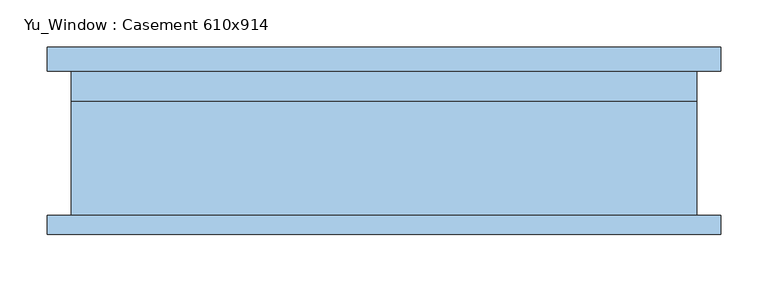
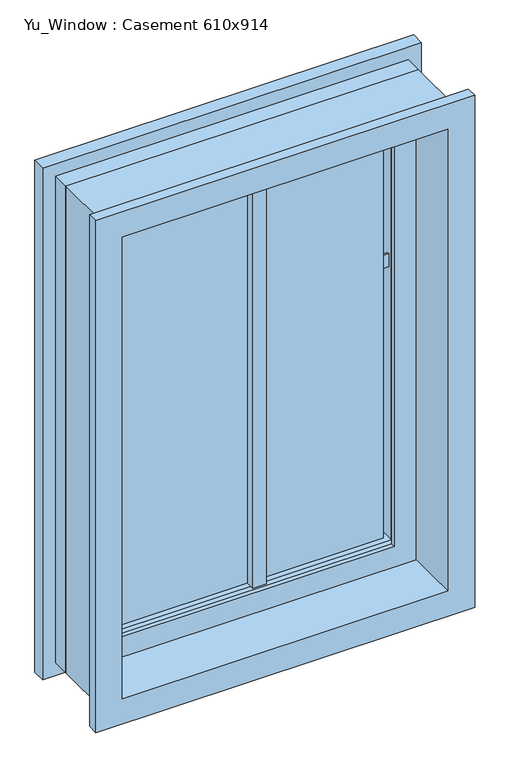
"""IFC4 building model written with IfcOpenShell, lengths in millimetres: window geometry, Yu_Window : Casement 610x914."""

from ifc_helpers import new_model, si_unit, frame, origin, place, context, project, spatial, polyline, outline, extrude, faceted_brep, source, transform, mapped, element, save


def yu_window_casement_610x914_cab7b646(model_context):
    return source(origin(), model_context, "Body", "SolidModel", [
        faceted_brep([(279.8, 23.8, 1489.4), (279.8, 43.8, 1489.4), (279.8, 43.8, 625.0), (279.8, 23.8, 625.0), (329.8, 43.8, 1539.4), (329.8, 43.8, 575.0), (-329.8, 43.8, 575.0), (-329.8, 43.8, 1539.4), (-279.8, 43.8, 1489.4), (-279.8, 43.8, 625.0), (-279.8, 23.8, 625.0), (-304.8, 23.8, 1514.4), (-304.8, 23.8, 600.0), (304.8, 23.8, 600.0), (304.8, 23.8, 1514.4), (-279.8, 23.8, 1489.4), (304.8, -96.2, 1514.4), (304.8, -96.2, 600.0), (-304.8, -96.2, 600.0), (-354.8, -96.2, 1564.4), (-354.8, -96.2, 550.0), (354.8, -96.2, 550.0), (354.8, -96.2, 1564.4), (-304.8, -96.2, 1514.4), (354.8, -76.2, 1564.4), (354.8, -76.2, 550.0), (-354.8, -76.2, 550.0), (-354.8, -76.2, 1564.4), (-329.8, -76.2, 1539.4), (-329.8, -76.2, 575.0), (329.8, -76.2, 575.0), (329.8, -76.2, 1539.4)], [[[0, 1, 2, 3]], [[4, 5, 6, 7], [8, 9, 2, 1]], [[3, 2, 9, 10]], [[11, 12, 13, 14], [0, 3, 10, 15]], [[16, 14, 13, 17]], [[17, 13, 12, 18]], [[19, 20, 21, 22], [16, 17, 18, 23]], [[24, 22, 21, 25]], [[25, 21, 20, 26]], [[24, 25, 26, 27], [28, 29, 30, 31]], [[4, 31, 30, 5]], [[5, 30, 29, 6]], [[10, 9, 8, 15]], [[18, 12, 11, 23]], [[26, 20, 19, 27]], [[6, 29, 28, 7]], [[15, 8, 1, 0]], [[23, 11, 14, 16]], [[27, 19, 22, 24]], [[7, 28, 31, 4]]]),
        faceted_brep([(-279.8, 68.8, 1489.4), (-279.8, 43.8, 1489.4), (-279.8, 43.8, 625.0), (-279.8, 68.8, 625.0), (-329.8, 43.8, 1539.4), (-329.8, 43.8, 575.0), (329.8, 43.8, 575.0), (329.8, 43.8, 1539.4), (279.8, 43.8, 1489.4), (279.8, 43.8, 625.0), (279.8, 68.8, 625.0), (304.8, 68.8, 1514.4), (304.8, 68.8, 600.0), (-304.8, 68.8, 600.0), (-304.8, 68.8, 1514.4), (279.8, 68.8, 1489.4), (-304.8, 101.2, 1514.4), (-304.8, 101.2, 600.0), (304.8, 101.2, 600.0), (354.8, 101.2, 1564.4), (354.8, 101.2, 550.0), (-354.8, 101.2, 550.0), (-354.8, 101.2, 1564.4), (304.8, 101.2, 1514.4), (-354.8, 76.2, 1564.4), (-354.8, 76.2, 550.0), (354.8, 76.2, 550.0), (354.8, 76.2, 1564.4), (329.8, 76.2, 1539.4), (329.8, 76.2, 575.0), (-329.8, 76.2, 575.0), (-329.8, 76.2, 1539.4)], [[[0, 1, 2, 3]], [[4, 5, 6, 7], [8, 9, 2, 1]], [[3, 2, 9, 10]], [[11, 12, 13, 14], [0, 3, 10, 15]], [[16, 14, 13, 17]], [[17, 13, 12, 18]], [[19, 20, 21, 22], [16, 17, 18, 23]], [[24, 22, 21, 25]], [[25, 21, 20, 26]], [[24, 25, 26, 27], [28, 29, 30, 31]], [[4, 31, 30, 5]], [[5, 30, 29, 6]], [[10, 9, 8, 15]], [[18, 12, 11, 23]], [[26, 20, 19, 27]], [[6, 29, 28, 7]], [[15, 8, 1, 0]], [[23, 11, 14, 16]], [[27, 19, 22, 24]], [[7, 28, 31, 4]]]),
        extrude(outline(polyline([(605.0, 299.8), (1509.4, 299.8), (1509.4, -299.8), (605.0, -299.8), (605.0, 299.8)]), holes=[polyline([(645.0, -259.8), (1469.4, -259.8), (1469.4, 259.8), (645.0, 259.8), (645.0, -259.8)])]), frame((0.0, 0.0, 0.0), z_axis=(0.0, 1.0, 0.0), x_axis=(0.0, 0.0, 1.0)), (0.0, 0.0, 1.0), 8.8),
        extrude(outline(polyline([(605.0, 299.8), (1509.4, 299.8), (1509.4, -299.8), (605.0, -299.8), (605.0, 299.8)]), holes=[polyline([(655.0, -249.8), (1459.4, -249.8), (1459.4, 249.8), (655.0, 249.8), (655.0, -249.8)])]), frame((0.0, 68.8, 0.0), z_axis=(0.0, 1.0, 0.0), x_axis=(0.0, 0.0, 1.0)), (0.0, 0.0, 1.0), 15.0),
        extrude(outline(polyline([(-249.8, 22.0), (249.8, 22.0), (249.8, 18.0), (-249.8, 18.0), (-249.8, 22.0)])), frame((0.0, 0.0, 655.0), z_axis=(0.0, 0.0, 1.0), x_axis=(1.0, 0.0, 0.0)), (0.0, 0.0, 1.0), 804.4),
        extrude(outline(polyline([(20.2, 68.8), (20.2, 0.0), (-4.8, 0.0), (-4.8, 68.8), (20.2, 68.8)])), frame((0.0, 0.0, 655.0), z_axis=(0.0, 0.0, 1.0), x_axis=(1.0, 0.0, 0.0)), (0.0, 0.0, 1.0), 854.4),
        extrude(outline(polyline([(-259.8, 18.0), (-259.8, 22.0), (259.8, 22.0), (259.8, 18.0), (-259.8, 18.0)])), frame((0.0, 0.0, 1189.4), z_axis=(0.0, 0.0, 1.0), x_axis=(1.0, 0.0, 0.0)), (0.0, 0.0, 1.0), 25.0),
    ])


if __name__ == "__main__":
    model = new_model("IFC4")
    model_context = context("Model", 3, world=origin())
    ifc_project = project(units=[si_unit("LENGTHUNIT", "METRE", prefix="MILLI")], contexts=[model_context])
    site = spatial("IfcSite", under=ifc_project)
    building = spatial("IfcBuilding", under=site)
    placement = place(None, origin())
    yu_window_casement_610x914_shape = yu_window_casement_610x914_cab7b646(model_context)
    element("IfcWindow", 1, ObjectType="Yu_Window : Casement 610x914", at=placement, inside=building, context=model_context, shape_type="MappedRepresentation", body=[
        mapped(yu_window_casement_610x914_shape, transform((0.0, 0.0, 0.0), x_axis=(1.0, 0.0, 0.0), y_axis=(0.0, 1.0, 0.0), z_axis=(0.0, 0.0, 1.0))),
    ])
    save(model, "model.ifc")

# Revit data of these elements
# Type "Yu_Window : Casement 610x914"
#   Type Mark = "24"
#   Analytic Construction = "<None>"
#   mullion 2 = 0' - 11.81102"
#   Window panel size 1 = 0' - 11.81102"
#   Offset = 0' - 0.98425"
#   Height = 3' - 0"
#   Default Sill Height = 1' - 11.62205"
#   Width = 2' - 0"
#   Define Thermal Properties by = 1
#   Interior material = none
#   Exterior material = none
#   Wall Closure = (empty or 0)
# Element 1 (IfcWindow, "Yu_Window : Casement 610x914")
#   Materials on its faces: "Glass"
# Materials
#   "Glass": class "Glass", colour RGB 0 128 192, transparency 0.75, Description = "Soda Lime Glass", Cost = 0
